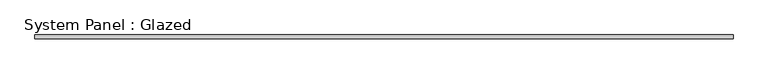
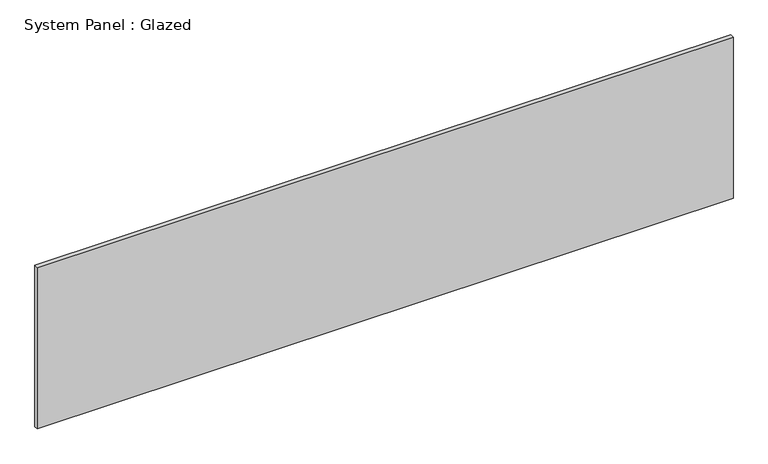
"""IFC4 building model written with IfcOpenShell, lengths in millimetres: plate geometry, System Panel : Glazed."""

from ifc_helpers import new_model, si_unit, origin, origin_with_axes, place, context, project, spatial, polyline, outline, extrude, source, transform, mapped, element, save


def system_panel_glazed_e5e35a93(model_context):
    return source(origin(), model_context, "Body", "SweptSolid", [
        extrude(outline(polyline([(2360.8752083, 19.05), (-2360.8752083, 19.05), (-2360.8752083, 44.45), (2360.8752083, 44.45), (2360.8752083, 19.05)])), origin_with_axes(), (0.0, 0.0, 1.0), 1155.7),
    ])


if __name__ == "__main__":
    model = new_model("IFC4")
    model_context = context("Model", 3, world=origin())
    ifc_project = project(units=[si_unit("LENGTHUNIT", "METRE", prefix="MILLI")], contexts=[model_context])
    site = spatial("IfcSite", under=ifc_project)
    building = spatial("IfcBuilding", under=site)
    placement = place(None, origin())
    system_panel_glazed_shape = system_panel_glazed_e5e35a93(model_context)
    element("IfcPlate", 1, ObjectType="System Panel : Glazed", at=placement, inside=building, context=model_context, shape_type="MappedRepresentation", body=[
        mapped(system_panel_glazed_shape, transform((0.0, 0.0, 0.0), x_axis=(1.0, 0.0, 0.0), y_axis=(0.0, 1.0, 0.0), z_axis=(0.0, 0.0, 1.0))),
    ])
    save(model, "model.ifc")

# Revit data of these elements
# Type "System Panel : Glazed"
#   Construction Type Id = "GSP4R"
#   Analytic Construction = "1/8 in Pilkington single glazing"
#   Visual Light Transmittance = 0.9
#   Solar Heat Gain Coefficient = 0.86
#   Heat Transfer Coefficient (U) = 1.18115 BTU/(h·ft²·°F)
# Element 1 (IfcPlate, "System Panel : Glazed")
#   Materials on its faces: "Glass"
# Materials
#   "Glass": class "Glass", colour RGB 0 128 192, transparency 0.75, Description = "Soda Lime Glass", Cost = 0
